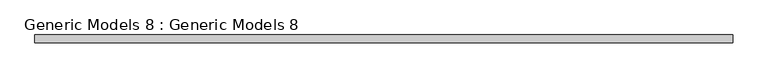
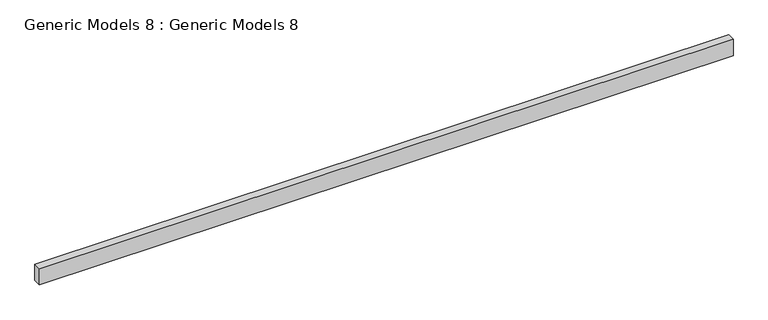
"""IFC4 building model written with IfcOpenShell, lengths in millimetres: proxy geometry, Generic Models 8 : Generic Models 8."""

from ifc_helpers import new_model, si_unit, frame, origin, place, context, project, spatial, polyline, outline, extrude, source, transform, mapped, element, save


def generic_models_8_generic_models_8_a9945552(model_context):
    return source(origin(), model_context, "Body", "SweptSolid", [
        extrude(outline(polyline([(12604.4370151, -3682.5004242), (12604.4370151, -3923.8847558), (-8934.7629849, -3923.8847558), (-8934.7629849, -3682.5004242), (12604.4370151, -3682.5004242)])), frame((0.0, 0.0, 19314.7959331), z_axis=(0.0, 0.0, 1.0), x_axis=(1.0, 0.0, 0.0)), (0.0, 0.0, 1.0), 533.5785966),
    ])


if __name__ == "__main__":
    model = new_model("IFC4")
    model_context = context("Model", 3, world=origin())
    ifc_project = project(units=[si_unit("LENGTHUNIT", "METRE", prefix="MILLI")], contexts=[model_context])
    site = spatial("IfcSite", under=ifc_project)
    building = spatial("IfcBuilding", under=site)
    placement = place(None, origin())
    generic_models_8_generic_models_8_shape = generic_models_8_generic_models_8_a9945552(model_context)
    element("IfcBuildingElementProxy", 1, Name="Generic Models 8 : Generic Models 8", ObjectType="Generic Models 8 : Generic Models 8", at=placement, inside=building, context=model_context, shape_type="MappedRepresentation", body=[
        mapped(generic_models_8_generic_models_8_shape, transform((0.0, 0.0, 0.0), x_axis=(1.0, 0.0, 0.0), y_axis=(0.0, 1.0, 0.0), z_axis=(0.0, 0.0, 1.0))),
    ])
    save(model, "model.ifc")
